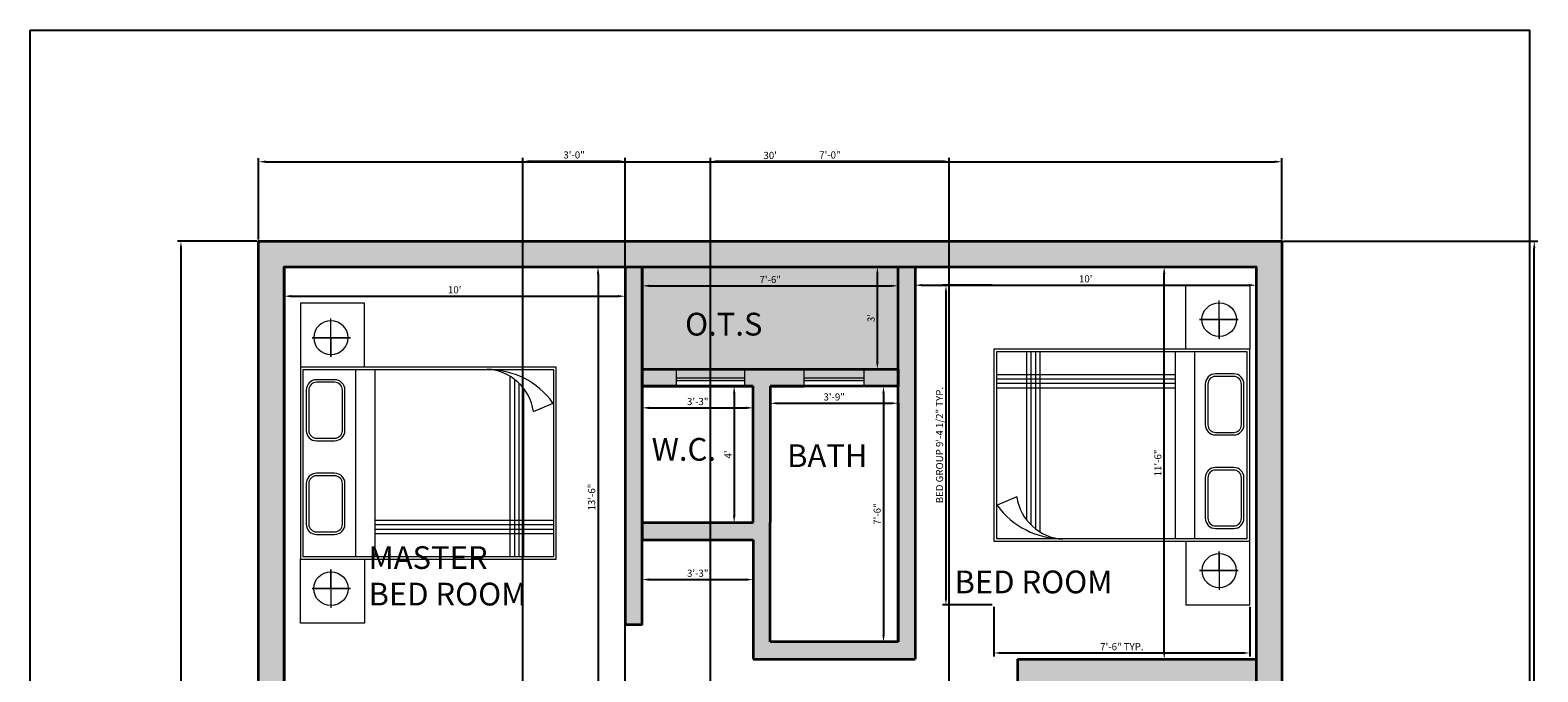
# Model space of a CAD drawing. Units: inches. Extents: x 2341 to 2872, y 1788 to 2419.
# Tile 3 of 3: x 2341 to 2872, y 2194 to 2419. Entities that reach past the tile are written whole.
import ezdxf

# ---------------------------------------------------------------- set-up
doc = ezdxf.new("R2010")
doc.units = ezdxf.units.IN
for name, color, linetype, lineweight in [('A-ANNO-DIMS', 2, 'Continuous', 18), ('A-ANNO-TTLB', 7, 'Continuous', 25), ('A-AREA-IDEN', 7, 'Continuous', 25), ('A-FURN', 8, 'Continuous', 18), ('A-GLAZ', 4, 'Continuous', 18), ('A-WALL', 7, 'Continuous', 35)]:
    doc.layers.add(name, color=color, linetype=linetype, lineweight=lineweight)
doc.layers.add('A-WALL-PATT', color=18, linetype='Continuous', lineweight=13, true_color=0x000000)
doc.styles.get("Standard").update_dxf_attribs({"font": 'arial.ttf'})
doc.dimstyles.new('Copy of ISO-25', dxfattribs={"dimtxt": 2.5, "dimasz": 2.5, "dimexe": 1.25, "dimexo": 0.625, "dimtad": 1, "dimdec": 1, "dimlunit": 4, "dimtxsty": 'Standard', "dimcen": 2.5, "dimadec": 0, "dimazin": 0, "dimtfac": 1, "dimtdec": 1, "dimtmove": 0, "dimatfit": 3, "dimfxl": 1, "dimarcsym": 0})

# ---------------------------------------------------------------- blocks, each defined once
blk = doc.blocks.new('*D1')
at = {"layer": 'A-ANNO-DIMS', "color": 0, "lineweight": -2, "transparency": 16777216}
for p, q in [((2421.55, 2345.64), (2421.55, 2374.26)), ((2424.05, 2373.01), (2779.05, 2373.01)), ((2781.55, 2345.64), (2781.55, 2374.26))]:
    blk.add_line(p, q, dxfattribs=at)
at = {"layer": 'A-ANNO-DIMS', "color": 0, "transparency": 16777216}
for points in [[(2424.05, 2373.43), (2424.05, 2372.6), (2421.55, 2373.01)], [(2779.05, 2373.43), (2779.05, 2372.6), (2781.55, 2373.01)]]:
    blk.add_solid(points, dxfattribs=at)
at = {"layer": 'Defpoints', "color": 0, "transparency": 16777216}
for p in [(2781.55, 2373.01), (2421.55, 2345.02), (2781.55, 2345.02)]:
    blk.add_point(p, dxfattribs=at)
at = {"layer": 'A-ANNO-DIMS', "color": 0, "transparency": 16777216, "insert": (2601.55, 2374.91), "char_height": 2.5, "attachment_point": 5}
blk.add_mtext("30'", dxfattribs=at)
blk = doc.blocks.new('A$C057D194F')
for p, q in [((0, 1.5, -0.169), (0, 2, -0.169)), ((0, 2, -0.169), (0.5, 2, -0.169)), ((0.269, 1.908, -0.169), (0.269, 1.761, -0.169)), ((0.269, 1.608, -0.169), (0.269, 1.908, -0.169)), ((0.5, 2, -0.169), (0.5, 0, -0.169)), ((2, 2, -0.169), (0.5, 2, -0.169)), ((1.98, 1.98, -0.169), (0.52, 1.98, -0.169)), ((0.52, 1.98, -0.169), (0.52, 0.02, -0.169)), ((1.091, 1.954, -0.169), (0.773, 1.954, -0.169)), ((1.091, 1.934, -0.169), (0.773, 1.934, -0.169)), ((1.822, 1.954, -0.169), (1.505, 1.954, -0.169)), ((1.822, 1.934, -0.169), (1.505, 1.934, -0.169)), ((1.98, 0.02, -0.169), (1.98, 1.98, -0.169)), ((2, 0, -0.169), (2, 2, -0.169)), ((2.5, 2, -0.169), (2, 2, -0.169)), ((2.231, 1.908, -0.169), (2.231, 1.761, -0.169)), ((2.231, 1.608, -0.169), (2.231, 1.908, -0.169)), ((2.5, 1.5, -0.169), (2.5, 2, -0.169)), ((0.693, 1.874, -0.169), (0.693, 1.732, -0.169)), ((0.713, 1.874, -0.169), (0.713, 1.732, -0.169)), ((1.151, 1.732, -0.169), (1.151, 1.874, -0.169)), ((1.171, 1.732, -0.169), (1.171, 1.874, -0.169)), ((1.425, 1.874, -0.169), (1.425, 1.732, -0.169)), ((1.445, 1.874, -0.169), (1.445, 1.732, -0.169)), ((1.882, 1.732, -0.169), (1.882, 1.874, -0.169)), ((1.902, 1.732, -0.169), (1.902, 1.874, -0.169)), ((0.419, 1.761, -0.169), (0.119, 1.761, -0.169)), ((0.269, 1.761, -0.169), (0.419, 1.761, -0.169)), ((0.269, 1.761, -0.169), (0.269, 1.608, -0.169)), ((0.773, 1.672, -0.169), (1.091, 1.672, -0.169)), ((0.773, 1.652, -0.169), (1.091, 1.652, -0.169)), ((1.505, 1.672, -0.169), (1.822, 1.672, -0.169)), ((1.505, 1.652, -0.169), (1.822, 1.652, -0.169)), ((2.081, 1.761, -0.169), (2.381, 1.761, -0.169)), ((2.231, 1.761, -0.169), (2.081, 1.761, -0.169)), ((2.231, 1.761, -0.169), (2.231, 1.608, -0.169)), ((1.98, 1.569, -0.169), (0.52, 1.569, -0.169)), ((0.5, 1.5, -0.169), (0, 1.5, -0.169)), ((1.98, 1.419, -0.169), (0.52, 1.419, -0.169)), ((0.697, 0.02, -0.169), (0.697, 1.419, -0.169)), ((0.732, 0.02, -0.169), (0.732, 1.419, -0.169)), ((0.767, 0.02, -0.169), (0.767, 1.419, -0.169)), ((0.802, 0.02, -0.169), (0.802, 1.419, -0.169)), ((2, 1.5, -0.169), (2.5, 1.5, -0.169)), ((0.52, 0.359, -0.169), (1.929, 0.359, -0.169)), ((0.52, 0.324, -0.169), (1.905, 0.324, -0.169)), ((0.52, 0.289, -0.169), (1.874, 0.289, -0.169)), ((0.52, 0.254, -0.169), (1.834, 0.254, -0.169)), ((1.655, 0.179, -0.169), (1.72, 0.025, -0.169)), ((0.52, 0.02, -0.169), (1.98, 0.02, -0.169)), ((0.5, 0, -0.169), (2, 0, -0.169))]:
    blk.add_line(p, q)
for centre, radius, start, end in [((0.773, 1.874, -0.169), 0.08, 90, 180), ((0.773, 1.874, -0.169), 0.06, 90, 180), ((1.091, 1.874, -0.169), 0.08, 0, 90), ((1.091, 1.874, -0.169), 0.06, 0, 90), ((1.505, 1.874, -0.169), 0.08, 90, 180), ((1.505, 1.874, -0.169), 0.06, 90, 180), ((1.822, 1.874, -0.169), 0.08, 0, 90), ((1.822, 1.874, -0.169), 0.06, 0, 90), ((0.773, 1.732, -0.169), 0.08, 180, 270), ((0.773, 1.732, -0.169), 0.06, 180, 270), ((1.091, 1.732, -0.169), 0.08, 270, 0), ((1.091, 1.732, -0.169), 0.06, 270, 0), ((1.505, 1.732, -0.169), 0.08, 180, 270), ((1.505, 1.732, -0.169), 0.06, 180, 270), ((1.822, 1.732, -0.169), 0.08, 270, 0), ((1.822, 1.732, -0.169), 0.06, 270, 0), ((1.599, 0.562, -0.169), 0.387, 278.2518, 356.6808), ((1.363, 0.529, -0.169), 0.617, 305.3295, 1.0459)]:
    blk.add_arc(centre, radius, start, end)
blk.add_ellipse((0.269, 1.761, -0.169), major_axis=(0, -0.135), ratio=0.975448)
at = {"extrusion": (0, 0, -1)}
blk.add_ellipse((2.231, 1.761, -0.169), major_axis=(0, 0.135), ratio=0.975448, dxfattribs=at)
for p in [(0.269, 1.761, -0.169), (2.231, 1.761, -0.169)]:
    blk.add_point(p)
blk = doc.blocks.new('*D4')
at = {"layer": 'A-ANNO-DIMS', "color": 0, "lineweight": -2, "transparency": 16777216}
for p, q in [((2420.93, 2345.02), (2392.99, 2345.02)), ((2394.24, 2342.52), (2394.24, 1987.52)), ((2420.93, 1985.02), (2392.99, 1985.02))]:
    blk.add_line(p, q, dxfattribs=at)
at = {"layer": 'A-ANNO-DIMS', "color": 0, "transparency": 16777216}
for points in [[(2393.82, 2342.52), (2394.66, 2342.52), (2394.24, 2345.02)], [(2393.82, 1987.52), (2394.66, 1987.52), (2394.24, 1985.02)]]:
    blk.add_solid(points, dxfattribs=at)
at = {"layer": 'Defpoints', "color": 0, "transparency": 16777216}
for p in [(2421.55, 2345.02), (2394.24, 1985.02), (2421.55, 1985.02)]:
    blk.add_point(p, dxfattribs=at)
at = {"layer": 'A-ANNO-DIMS', "color": 0, "transparency": 16777216, "insert": (2392.34, 2165.02), "char_height": 2.5, "attachment_point": 5, "rotation": 90}
blk.add_mtext("30'", dxfattribs=at)
blk = doc.blocks.new('*D7')
at = {"layer": 'A-ANNO-DIMS', "color": 0, "lineweight": -2, "transparency": 16777216}
for p, q in [((2430.55, 2335.39), (2430.55, 2324.45)), ((2550.55, 2335.39), (2550.55, 2324.45)), ((2433.05, 2325.7), (2548.05, 2325.7))]:
    blk.add_line(p, q, dxfattribs=at)
at = {"layer": 'A-ANNO-DIMS', "color": 0, "transparency": 16777216}
for points in [[(2433.05, 2326.12), (2433.05, 2325.29), (2430.55, 2325.7)], [(2548.05, 2326.12), (2548.05, 2325.29), (2550.55, 2325.7)]]:
    blk.add_solid(points, dxfattribs=at)
at = {"layer": 'Defpoints', "color": 0, "transparency": 16777216}
for p in [(2430.55, 2336.02), (2550.55, 2336.02), (2550.55, 2325.7)]:
    blk.add_point(p, dxfattribs=at)
at = {"layer": 'A-ANNO-DIMS', "color": 0, "transparency": 16777216, "insert": (2490.55, 2327.61), "char_height": 2.5, "attachment_point": 5}
blk.add_mtext("10'", dxfattribs=at)
blk = doc.blocks.new('*D8')
at = {"layer": 'A-ANNO-DIMS', "color": 0, "lineweight": -2, "transparency": 16777216}
for p, q in [((2549.93, 2336.02), (2539.72, 2336.02)), ((2540.97, 2333.52), (2540.97, 2176.52)), ((2549.93, 2174.02), (2539.72, 2174.02))]:
    blk.add_line(p, q, dxfattribs=at)
at = {"layer": 'A-ANNO-DIMS', "color": 0, "transparency": 16777216}
for points in [[(2540.56, 2333.52), (2541.39, 2333.52), (2540.97, 2336.02)], [(2540.56, 2176.52), (2541.39, 2176.52), (2540.97, 2174.02)]]:
    blk.add_solid(points, dxfattribs=at)
at = {"layer": 'Defpoints', "color": 0, "transparency": 16777216}
for p in [(2550.55, 2336.02), (2540.97, 2174.02), (2550.55, 2174.02)]:
    blk.add_point(p, dxfattribs=at)
at = {"layer": 'A-ANNO-DIMS', "color": 0, "transparency": 16777216, "insert": (2539.07, 2255.02), "char_height": 2.5, "attachment_point": 5, "rotation": 90}
blk.add_mtext('13\'-6"', dxfattribs=at)
blk = doc.blocks.new('*D9')
at = {"layer": 'A-ANNO-DIMS', "color": 0, "lineweight": -2, "transparency": 16777216}
for p, q in [((2556.55, 2335.39), (2556.55, 2328.09)), ((2646.55, 2335.39), (2646.55, 2328.09)), ((2559.05, 2329.34), (2644.05, 2329.34))]:
    blk.add_line(p, q, dxfattribs=at)
at = {"layer": 'A-ANNO-DIMS', "color": 0, "transparency": 16777216}
for points in [[(2559.05, 2329.76), (2559.05, 2328.93), (2556.55, 2329.34)], [(2644.05, 2329.76), (2644.05, 2328.93), (2646.55, 2329.34)]]:
    blk.add_solid(points, dxfattribs=at)
at = {"layer": 'Defpoints', "color": 0, "transparency": 16777216}
for p in [(2556.55, 2336.02), (2646.55, 2336.02), (2646.55, 2329.34)]:
    blk.add_point(p, dxfattribs=at)
at = {"layer": 'A-ANNO-DIMS', "color": 0, "transparency": 16777216, "insert": (2601.55, 2331.24), "char_height": 2.5, "attachment_point": 5}
blk.add_mtext('7\'-6"', dxfattribs=at)
blk = doc.blocks.new('*D10')
at = {"layer": 'A-ANNO-DIMS', "color": 0, "lineweight": -2, "transparency": 16777216}
for p, q in [((2645.93, 2336.02), (2638.01, 2336.02)), ((2639.26, 2302.52), (2639.26, 2333.52)), ((2645.93, 2300.02), (2638.01, 2300.02))]:
    blk.add_line(p, q, dxfattribs=at)
at = {"layer": 'A-ANNO-DIMS', "color": 0, "transparency": 16777216}
for points in [[(2638.84, 2333.52), (2639.67, 2333.52), (2639.26, 2336.02)], [(2638.84, 2302.52), (2639.67, 2302.52), (2639.26, 2300.02)]]:
    blk.add_solid(points, dxfattribs=at)
at = {"layer": 'Defpoints', "color": 0, "transparency": 16777216}
for p in [(2639.26, 2336.02), (2646.55, 2336.02), (2646.55, 2300.02)]:
    blk.add_point(p, dxfattribs=at)
at = {"layer": 'A-ANNO-DIMS', "color": 0, "transparency": 16777216, "insert": (2637.36, 2318.02), "char_height": 2.5, "attachment_point": 5, "rotation": 90}
blk.add_mtext("3'", dxfattribs=at)
blk = doc.blocks.new('*D11')
at = {"layer": 'A-ANNO-DIMS', "color": 0, "lineweight": -2, "transparency": 16777216}
for p, q in [((2601.55, 2293.39), (2601.55, 2286.77)), ((2646.55, 2293.39), (2646.55, 2286.77)), ((2604.05, 2288.02), (2644.05, 2288.02))]:
    blk.add_line(p, q, dxfattribs=at)
at = {"layer": 'A-ANNO-DIMS', "color": 0, "transparency": 16777216}
for points in [[(2604.05, 2288.43), (2604.05, 2287.6), (2601.55, 2288.02)], [(2644.05, 2288.43), (2644.05, 2287.6), (2646.55, 2288.02)]]:
    blk.add_solid(points, dxfattribs=at)
at = {"layer": 'Defpoints', "color": 0, "transparency": 16777216}
for p in [(2601.55, 2294.02), (2646.55, 2294.02), (2646.55, 2288.02)]:
    blk.add_point(p, dxfattribs=at)
at = {"layer": 'A-ANNO-DIMS', "color": 0, "transparency": 16777216, "insert": (2624.05, 2289.92), "char_height": 2.5, "attachment_point": 5}
blk.add_mtext('3\'-9"', dxfattribs=at)
blk = doc.blocks.new('*D12')
at = {"layer": 'A-ANNO-DIMS', "color": 0, "lineweight": -2, "transparency": 16777216}
for p, q in [((2645.93, 2294.02), (2640.16, 2294.02)), ((2641.41, 2291.52), (2641.41, 2206.52)), ((2645.93, 2204.02), (2640.16, 2204.02))]:
    blk.add_line(p, q, dxfattribs=at)
at = {"layer": 'A-ANNO-DIMS', "color": 0, "transparency": 16777216}
for points in [[(2640.99, 2291.52), (2641.82, 2291.52), (2641.41, 2294.02)], [(2640.99, 2206.52), (2641.82, 2206.52), (2641.41, 2204.02)]]:
    blk.add_solid(points, dxfattribs=at)
at = {"layer": 'Defpoints', "color": 0, "transparency": 16777216}
for p in [(2646.55, 2294.02), (2641.41, 2204.02), (2646.55, 2204.02)]:
    blk.add_point(p, dxfattribs=at)
at = {"layer": 'A-ANNO-DIMS', "color": 0, "transparency": 16777216, "insert": (2639.5, 2249.02), "char_height": 2.5, "attachment_point": 5, "rotation": 90}
blk.add_mtext('7\'-6"', dxfattribs=at)
blk = doc.blocks.new('*D13')
at = {"layer": 'A-ANNO-DIMS', "color": 0, "lineweight": -2, "transparency": 16777216}
for p, q in [((2556.55, 2293.39), (2556.55, 2285.16)), ((2595.55, 2293.39), (2595.55, 2285.16)), ((2559.05, 2286.41), (2593.05, 2286.41))]:
    blk.add_line(p, q, dxfattribs=at)
at = {"layer": 'A-ANNO-DIMS', "color": 0, "transparency": 16777216}
for points in [[(2559.05, 2286.83), (2559.05, 2285.99), (2556.55, 2286.41)], [(2593.05, 2286.83), (2593.05, 2285.99), (2595.55, 2286.41)]]:
    blk.add_solid(points, dxfattribs=at)
at = {"layer": 'Defpoints', "color": 0, "transparency": 16777216}
for p in [(2556.55, 2294.02), (2595.55, 2294.02), (2595.55, 2286.41)]:
    blk.add_point(p, dxfattribs=at)
at = {"layer": 'A-ANNO-DIMS', "color": 0, "transparency": 16777216, "insert": (2576.05, 2288.31), "char_height": 2.5, "attachment_point": 5}
blk.add_mtext('3\'-3"', dxfattribs=at)
blk = doc.blocks.new('*D14')
at = {"layer": 'A-ANNO-DIMS', "color": 0, "lineweight": -2, "transparency": 16777216}
for p, q in [((2594.93, 2294.02), (2587.63, 2294.02)), ((2588.88, 2291.52), (2588.88, 2248.52)), ((2594.93, 2246.02), (2587.63, 2246.02))]:
    blk.add_line(p, q, dxfattribs=at)
at = {"layer": 'A-ANNO-DIMS', "color": 0, "transparency": 16777216}
for points in [[(2588.46, 2291.52), (2589.3, 2291.52), (2588.88, 2294.02)], [(2588.46, 2248.52), (2589.3, 2248.52), (2588.88, 2246.02)]]:
    blk.add_solid(points, dxfattribs=at)
at = {"layer": 'Defpoints', "color": 0, "transparency": 16777216}
for p in [(2595.55, 2294.02), (2588.88, 2246.02), (2595.55, 2246.02)]:
    blk.add_point(p, dxfattribs=at)
at = {"layer": 'A-ANNO-DIMS', "color": 0, "transparency": 16777216, "insert": (2587.01, 2270.02), "char_height": 2.5, "attachment_point": 5, "rotation": 90}
blk.add_mtext("4'", dxfattribs=at)
blk = doc.blocks.new('*D15')
at = {"layer": 'A-ANNO-DIMS', "color": 0, "lineweight": -2, "transparency": 16777216}
for p, q in [((2652.55, 2335.39), (2652.55, 2328.32)), ((2772.55, 2335.39), (2772.55, 2328.32)), ((2655.05, 2329.57), (2770.05, 2329.57))]:
    blk.add_line(p, q, dxfattribs=at)
at = {"layer": 'A-ANNO-DIMS', "color": 0, "transparency": 16777216}
for points in [[(2655.05, 2329.98), (2655.05, 2329.15), (2652.55, 2329.57)], [(2770.05, 2329.98), (2770.05, 2329.15), (2772.55, 2329.57)]]:
    blk.add_solid(points, dxfattribs=at)
at = {"layer": 'Defpoints', "color": 0, "transparency": 16777216}
for p in [(2652.55, 2336.02), (2772.55, 2336.02), (2772.55, 2329.57)]:
    blk.add_point(p, dxfattribs=at)
at = {"layer": 'A-ANNO-DIMS', "color": 0, "transparency": 16777216, "insert": (2712.55, 2331.47), "char_height": 2.5, "attachment_point": 5}
blk.add_mtext("10'", dxfattribs=at)
blk = doc.blocks.new('*D16')
at = {"layer": 'A-ANNO-DIMS', "color": 0, "lineweight": -2, "transparency": 16777216}
for p, q in [((2771.93, 2336.02), (2738.91, 2336.02)), ((2740.16, 2200.52), (2740.16, 2333.52)), ((2771.93, 2198.02), (2738.91, 2198.02))]:
    blk.add_line(p, q, dxfattribs=at)
at = {"layer": 'A-ANNO-DIMS', "color": 0, "transparency": 16777216}
for points in [[(2739.74, 2333.52), (2740.58, 2333.52), (2740.16, 2336.02)], [(2739.74, 2200.52), (2740.58, 2200.52), (2740.16, 2198.02)]]:
    blk.add_solid(points, dxfattribs=at)
at = {"layer": 'Defpoints', "color": 0, "transparency": 16777216}
for p in [(2740.16, 2336.02), (2772.55, 2336.02), (2772.55, 2198.02)]:
    blk.add_point(p, dxfattribs=at)
at = {"layer": 'A-ANNO-DIMS', "color": 0, "transparency": 16777216, "insert": (2738.26, 2267.02), "char_height": 2.5, "attachment_point": 5, "rotation": 90}
blk.add_mtext('11\'-6"', dxfattribs=at)
blk = doc.blocks.new('*D29')
at = {"layer": 'A-ANNO-DIMS', "color": 0, "lineweight": -2, "transparency": 16777216}
for p, q in [((2556.55, 2239.39), (2556.55, 2224.73)), ((2595.55, 2239.39), (2595.55, 2224.73)), ((2559.05, 2225.98), (2593.05, 2225.98))]:
    blk.add_line(p, q, dxfattribs=at)
at = {"layer": 'A-ANNO-DIMS', "color": 0, "transparency": 16777216}
for points in [[(2559.05, 2226.4), (2559.05, 2225.56), (2556.55, 2225.98)], [(2593.05, 2226.4), (2593.05, 2225.56), (2595.55, 2225.98)]]:
    blk.add_solid(points, dxfattribs=at)
at = {"layer": 'Defpoints', "color": 0, "transparency": 16777216}
for p in [(2556.55, 2240.02), (2595.55, 2240.02), (2595.55, 2225.98)]:
    blk.add_point(p, dxfattribs=at)
at = {"layer": 'A-ANNO-DIMS', "color": 0, "transparency": 16777216, "insert": (2576.05, 2227.88), "char_height": 2.5, "attachment_point": 5}
blk.add_mtext('3\'-3"', dxfattribs=at)
blk = doc.blocks.new('*D31')
at = {"layer": 'A-ANNO-DIMS', "color": 0, "lineweight": -2, "transparency": 16777216}
for p, q in [((2679.63, 2329.57), (2662.13, 2329.57)), ((2663.38, 2327.07), (2663.38, 2219.54)), ((2679.63, 2217.04), (2662.13, 2217.04))]:
    blk.add_line(p, q, dxfattribs=at)
at = {"layer": 'A-ANNO-DIMS', "color": 0, "transparency": 16777216}
for points in [[(2662.96, 2327.07), (2663.79, 2327.07), (2663.38, 2329.57)], [(2662.96, 2219.54), (2663.79, 2219.54), (2663.38, 2217.04)]]:
    blk.add_solid(points, dxfattribs=at)
at = {"layer": 'Defpoints', "color": 0, "transparency": 16777216}
for p in [(2680.26, 2329.57), (2663.38, 2217.04), (2680.26, 2217.04)]:
    blk.add_point(p, dxfattribs=at)
at = {"layer": 'A-ANNO-DIMS', "color": 0, "transparency": 16777216, "insert": (2661.46, 2273.3), "char_height": 2.5, "attachment_point": 5, "rotation": 90}
blk.add_mtext('BED GROUP 9\'-4 1/2" TYP.', dxfattribs=at)
blk = doc.blocks.new('*D32')
at = {"layer": 'A-ANNO-DIMS', "color": 0, "lineweight": -2, "transparency": 16777216}
for p, q in [((2680.26, 2216.41), (2680.26, 2198.91)), ((2770.28, 2216.41), (2770.28, 2198.91)), ((2682.76, 2200.16), (2767.78, 2200.16))]:
    blk.add_line(p, q, dxfattribs=at)
at = {"layer": 'A-ANNO-DIMS', "color": 0, "transparency": 16777216}
for points in [[(2682.76, 2200.57), (2682.76, 2199.74), (2680.26, 2200.16)], [(2767.78, 2200.57), (2767.78, 2199.74), (2770.28, 2200.16)]]:
    blk.add_solid(points, dxfattribs=at)
at = {"layer": 'Defpoints', "color": 0, "transparency": 16777216}
for p in [(2680.26, 2217.04), (2770.28, 2217.04), (2770.28, 2200.16)]:
    blk.add_point(p, dxfattribs=at)
at = {"layer": 'A-ANNO-DIMS', "color": 0, "transparency": 16777216, "insert": (2725.27, 2202.06), "char_height": 2.5, "attachment_point": 5}
blk.add_mtext('7\'-6" TYP.', dxfattribs=at)
blk = doc.blocks.new('*D35')
at = {"layer": 'A-ANNO-DIMS', "color": 0, "lineweight": -2, "transparency": 16777216}
for p, q in [((2782.18, 2345.02), (2871.62, 2345.02)), ((2870.37, 1945.52), (2870.37, 2342.52)), ((2782.18, 1943.02), (2871.62, 1943.02))]:
    blk.add_line(p, q, dxfattribs=at)
at = {"layer": 'A-ANNO-DIMS', "color": 0, "transparency": 16777216}
for points in [[(2869.95, 2342.52), (2870.78, 2342.52), (2870.37, 2345.02)], [(2869.95, 1945.52), (2870.78, 1945.52), (2870.37, 1943.02)]]:
    blk.add_solid(points, dxfattribs=at)
at = {"layer": 'Defpoints', "color": 0, "transparency": 16777216}
for p in [(2781.55, 2345.02), (2870.37, 2345.02), (2781.55, 1943.02)]:
    blk.add_point(p, dxfattribs=at)
at = {"layer": 'A-ANNO-DIMS', "color": 0, "transparency": 16777216, "insert": (2868.46, 2144.02), "char_height": 2.5, "attachment_point": 5, "rotation": 90}
blk.add_mtext('33\'-6"', dxfattribs=at)
blk = doc.blocks.new('*D37')
at = {"layer": 'A-ANNO-DIMS', "color": 0, "lineweight": -2, "transparency": 16777216}
for p, q in [((2580.55, 2120.64), (2580.55, 2374.42)), ((2583.05, 2373.17), (2662.05, 2373.17)), ((2664.55, 2120.64), (2664.55, 2374.42))]:
    blk.add_line(p, q, dxfattribs=at)
at = {"layer": 'A-ANNO-DIMS', "color": 0, "transparency": 16777216}
for points in [[(2583.05, 2373.58), (2583.05, 2372.75), (2580.55, 2373.17)], [(2662.05, 2373.58), (2662.05, 2372.75), (2664.55, 2373.17)]]:
    blk.add_solid(points, dxfattribs=at)
at = {"layer": 'Defpoints', "color": 0, "transparency": 16777216}
for p in [(2664.55, 2373.17), (2580.55, 2120.02), (2664.55, 2120.02)]:
    blk.add_point(p, dxfattribs=at)
at = {"layer": 'A-ANNO-DIMS', "color": 0, "transparency": 16777216, "insert": (2622.55, 2375.07), "char_height": 2.5, "attachment_point": 5}
blk.add_mtext('7\'-0"', dxfattribs=at)
blk = doc.blocks.new('*D38')
at = {"layer": 'A-ANNO-DIMS', "color": 0, "lineweight": -2, "transparency": 16777216}
for p, q in [((2514.55, 2120.64), (2514.55, 2374.42)), ((2517.05, 2373.17), (2548.05, 2373.17)), ((2550.55, 2120.64), (2550.55, 2374.42))]:
    blk.add_line(p, q, dxfattribs=at)
at = {"layer": 'A-ANNO-DIMS', "color": 0, "transparency": 16777216}
for points in [[(2517.05, 2373.58), (2517.05, 2372.75), (2514.55, 2373.17)], [(2548.05, 2373.58), (2548.05, 2372.75), (2550.55, 2373.17)]]:
    blk.add_solid(points, dxfattribs=at)
at = {"layer": 'Defpoints', "color": 0, "transparency": 16777216}
for p in [(2550.55, 2373.17), (2514.55, 2120.02), (2550.55, 2120.02)]:
    blk.add_point(p, dxfattribs=at)
at = {"layer": 'A-ANNO-DIMS', "color": 0, "transparency": 16777216, "insert": (2532.55, 2375.07), "char_height": 2.5, "attachment_point": 5}
blk.add_mtext('3\'-0"', dxfattribs=at)

msp = doc.modelspace()

# ---------------------------------------------------------------- hatches: boundary and pattern name
at = {"layer": 'A-WALL-PATT'}
h = msp.add_hatch(color=256, dxfattribs=at)
h.dxf.hatch_style = 1
h.paths.add_polyline_path([(2781.55, 2345.02), (2421.55, 2345.02), (2421.55, 1985.02), (2421.55, 1949.02), (2421.55, 1943.02), (2781.55, 1943.02), (2781.55, 1985.02)])
h.paths.add_polyline_path([(2550.55, 2336.02), (2772.55, 2336.02), (2772.55, 1994.02), (2772.55, 1985.02), (2772.55, 1947.02), (2430.55, 1947.02), (2430.55, 1985.02), (2454.55, 1985.02), (2454.55, 1994.02), (2430.55, 1994.02), (2430.55, 2114.02), (2496.55, 2114.02), (2514.55, 2114.02), (2514.55, 2120.02), (2496.55, 2120.02), (2496.55, 2168.02), (2556.55, 2168.02), (2556.55, 2174.02), (2550.55, 2174.02), (2478.55, 2174.02), (2478.55, 2170.02), (2490.55, 2170.02), (2490.55, 2168.02), (2490.55, 2120.02), (2430.55, 2120.02), (2430.55, 2168.02), (2430.55, 2174.02), (2430.55, 2204.02), (2430.55, 2336.02)], flags=16)
h.paths.add_polyline_path([(2556.55, 2336.02), (2652.55, 2336.02), (2652.55, 2198.02), (2646.55, 2198.02), (2601.55, 2198.02), (2595.55, 2198.02), (2595.55, 2240.02), (2556.55, 2240.02), (2556.55, 2246.02), (2556.55, 2294.02)], flags=0)
h.paths.add_polyline_path([(2556.55, 2300.02), (2646.55, 2300.02), (2646.55, 2294.02), (2646.55, 2204.02), (2601.55, 2204.02), (2601.55, 2246.02), (2601.55, 2294.02), (2613.55, 2294.02), (2613.55, 2300.02), (2592.55, 2300.02), (2592.55, 2294.02), (2595.55, 2294.02), (2595.55, 2246.02), (2556.55, 2246.02), (2556.55, 2282.02)], flags=0)
h.paths.add_polyline_path([(2680.26, 2307.06), (2747.77, 2307.06), (2747.77, 2329.57), (2770.28, 2329.57), (2770.28, 2307.06), (2770.28, 2239.54), (2770.28, 2217.04), (2747.77, 2217.04), (2747.77, 2239.54), (2680.26, 2239.54)], flags=0)
h.paths.add_polyline_path([(2681.16, 2306.16), (2769.38, 2306.16), (2769.38, 2240.44), (2704.56, 2240.44, -0.009128), (2703.54, 2240.44), (2681.16, 2240.44)], flags=0)
h.paths.add_polyline_path([(2744.14, 2298.19), (2744.14, 2293.47), (2696.44, 2293.47), (2696.44, 2242.73, -0.092104), (2691.71, 2247), (2691.71, 2298.19)], flags=0)
h.paths.add_polyline_path([(2694.86, 2296.62), (2694.86, 2295.04), (2693.29, 2295.04), (2693.29, 2296.62)], flags=0)
h.paths.add_polyline_path([(2478.55, 2173.02), (2478.55, 2172.02), (2478.55, 2171.02), (2442.55, 2171.02), (2442.55, 2170.02), (2438.98, 2170.02), (2430.55, 2170.02), (2430.55, 2174.02), (2442.55, 2174.02), (2442.55, 2173.02)], flags=0)
h.paths.add_polyline_path([(2688.55, 2198.02), (2697.55, 2198.02), (2772.55, 2198.02), (2772.55, 2189.02), (2772.55, 2153.02), (2755.26, 2153.02), (2755.26, 2145.02), (2772.55, 2145.02), (2772.55, 2137.02), (2755.26, 2137.02), (2755.26, 2129.02), (2772.55, 2129.02), (2772.55, 2121.02), (2755.26, 2121.02), (2755.26, 2119.07), (2757.66, 2119.07), (2755.26, 2113.02), (2772.55, 2113.02), (2772.55, 2105.02), (2736.55, 2105.02), (2736.55, 2153.02), (2697.55, 2153.02), (2697.55, 2021.02), (2697.55, 1952.02), (2688.89, 1952.02), (2688.89, 1947.02), (2688.59, 2021.02), (2688.55, 2021.02), (2580.55, 2021.02), (2580.55, 2030.02), (2556.55, 2030.02), (2556.55, 2114.02), (2580.55, 2114.02), (2580.55, 2120.02), (2664.55, 2120.02), (2688.55, 2120.02), (2688.55, 2189.02)], flags=0)
h.paths.add_polyline_path([(2510.86, 2109.17, -0.414214), (2512.75, 2107.25), (2512.59, 2085.13, -0.414214), (2511.43, 2083.99), (2508, 2084.02, -0.414214), (2506.86, 2085.17), (2487.78, 2085.31, -0.414214), (2485.88, 2087.24, -0.414214), (2483.96, 2085.34), (2464.87, 2085.49, -0.414214), (2462.98, 2087.41, -0.414214), (2461.06, 2085.52), (2441.97, 2085.66, -0.414214), (2440.82, 2084.52), (2437.38, 2084.55, -0.414214), (2436.25, 2085.7), (2436.41, 2107.83, -0.414214), (2438.34, 2109.72)], flags=0)
h.paths.add_polyline_path([(2736.55, 2189.02), (2736.55, 2170), (2728.55, 2170), (2728.55, 2153.02), (2720.55, 2153.02), (2720.55, 2189.02), (2712.55, 2189.02), (2712.55, 2153.02), (2704.55, 2153.02), (2704.55, 2189.02)], flags=0)
edge = h.paths.add_edge_path(flags=0)
edge.add_ellipse((2759.52, 2317.47), major_axis=(6.08, 0), ratio=0.975448, start_angle=450, end_angle=540, ccw=False)
edge.add_ellipse((2759.52, 2317.47), major_axis=(6.08, 0), ratio=0.975448, start_angle=360, end_angle=450, ccw=False)
edge.add_ellipse((2759.52, 2317.47), major_axis=(6.08, 0), ratio=0.975448, start_angle=270, end_angle=360, ccw=False)
edge.add_ellipse((2759.52, 2317.47), major_axis=(6.08, 0), ratio=0.975448, start_angle=180, end_angle=270, ccw=False)
h.paths.add_polyline_path([(2505.86, 2104.26, -0.414214), (2507, 2103.11), (2506.89, 2089.02), (2442, 2089.51), (2442.11, 2103.6, -0.414214), (2443.26, 2104.74)], flags=0)
h.paths.add_polyline_path([(2485.9, 2089.94), (2463, 2090.11), (2463.01, 2091.64), (2485.91, 2091.47)], flags=0)
h.paths.add_polyline_path([(2758.23, 2298.35), (2764.61, 2298.35, -0.414214), (2768.21, 2294.75), (2768.21, 2280.47, -0.414214), (2764.61, 2276.87), (2758.23, 2276.87, -0.414214), (2754.62, 2280.47), (2754.62, 2294.75, -0.414214)], flags=0)
h.paths.add_polyline_path([(2758.23, 2297.45), (2764.61, 2297.45, -0.414214), (2767.31, 2294.75), (2767.31, 2280.47, -0.414214), (2764.61, 2277.77), (2758.23, 2277.77, -0.414214), (2755.52, 2280.47), (2755.52, 2294.75, -0.414214)], flags=0)
h.paths.add_polyline_path([(2758.23, 2265.42), (2764.61, 2265.42, -0.414214), (2768.21, 2261.82), (2768.21, 2247.53, -0.414214), (2764.61, 2243.93), (2758.23, 2243.93, -0.414214), (2754.62, 2247.53), (2754.62, 2261.82, -0.414214)], flags=0)
h.paths.add_polyline_path([(2758.23, 2264.52), (2764.61, 2264.52, -0.414214), (2767.31, 2261.82), (2767.31, 2247.53, -0.414214), (2764.61, 2244.83), (2758.23, 2244.83, -0.414214), (2755.52, 2247.53), (2755.52, 2261.82, -0.414214)], flags=0)
edge = h.paths.add_edge_path(flags=0)
edge.add_ellipse((2759.52, 2229.13), major_axis=(6.08, 0), ratio=0.975448, start_angle=90, end_angle=180, ccw=False)
edge.add_ellipse((2759.52, 2229.13), major_axis=(6.08, 0), ratio=0.975448, start_angle=0, end_angle=90, ccw=False)
edge.add_ellipse((2759.52, 2229.13), major_axis=(6.08, 0), ratio=0.975448, start_angle=270, end_angle=360, ccw=False)
edge.add_ellipse((2759.52, 2229.13), major_axis=(6.08, 0), ratio=0.975448, start_angle=180, end_angle=270, ccw=False)
h.paths.add_polyline_path([(2457.94, 2073.59, -0.414214), (2459.08, 2072.44), (2459.05, 2069, -0.414214), (2457.9, 2067.87), (2457.75, 2048.78, -0.414214), (2455.83, 2046.89, -0.414214), (2457.72, 2044.96), (2457.58, 2025.88, -0.414214), (2455.66, 2023.98, -0.414214), (2457.55, 2022.06), (2457.41, 2002.98, -0.414214), (2458.54, 2001.82), (2458.52, 1998.39, -0.414214), (2457.36, 1997.25), (2435.24, 1997.42, -0.414214), (2433.35, 1999.34), (2433.89, 2071.86, -0.414214), (2435.82, 2073.76)], flags=0)
h.paths.add_polyline_path([(2454.05, 2067.89), (2453.56, 2003), (2439.47, 2003.11, -0.414214), (2438.33, 2004.26), (2438.8, 2066.86, -0.414214), (2439.96, 2068)], flags=0)
h.paths.add_polyline_path([(2452.95, 2024), (2451.43, 2024.02), (2451.6, 2046.92), (2453.13, 2046.91)], flags=0)
h.paths.add_polyline_path([(2830.4, 1819.46), (2838.99, 1819.46), (2838.99, 1828.46), (2830.4, 1828.46)], flags=9)
h.paths.add_polyline_path([(2814.93, 1841.19), (2823.62, 1841.19), (2823.62, 1850.5), (2814.93, 1850.5)], flags=9)
h.paths.add_polyline_path([(2843.19, 1840.36), (2852.25, 1840.36), (2852.25, 1849.36), (2843.19, 1849.36)], flags=9)
h.paths.add_polyline_path([(2828.19, 1854.15), (2839.1, 1854.15), (2839.1, 1863.15), (2828.19, 1863.15)], flags=9)
h.paths.add_polyline_path([(2760.12, 1830.89), (2792.1, 1830.89), (2792.1, 1840.21), (2760.12, 1840.21)], flags=9)
h.paths.add_polyline_path([(2760.12, 1840.53), (2800.48, 1840.53), (2800.48, 1849.85), (2760.12, 1849.85)], flags=9)
h.paths.add_polyline_path([(2758.73, 1854.24), (2815.82, 1854.24), (2815.82, 1863.56), (2758.73, 1863.56)], flags=9)
h.paths.add_polyline_path([(2482.08, 1917.73), (2536.72, 1917.73), (2536.72, 1936.36), (2482.08, 1936.36)], flags=9)
h.paths.add_polyline_path([(2707.72, 1951.32), (2770.13, 1951.32), (2770.13, 1963.73), (2707.72, 1963.73)], flags=8)
h.paths.add_polyline_path([(2706.05, 2121.97), (2725.65, 2121.97), (2725.65, 2134.17), (2706.05, 2134.17)], flags=8)
h.paths.add_polyline_path([(2705.12, 1972.11), (2749.62, 1972.11), (2749.62, 1984.52), (2705.12, 1984.52)], flags=8)
h.paths.add_polyline_path([(2468.66, 1961.36), (2524.36, 1961.36), (2524.36, 1973.77), (2468.66, 1973.77)], flags=8)
h.paths.add_polyline_path([(2572.95, 1988.2), (2639.05, 1988.2), (2639.05, 2000.2), (2572.95, 2000.2)], flags=8)
h.paths.add_polyline_path([(2460.85, 2050.66), (2556.87, 2050.66), (2556.87, 2063.08), (2460.85, 2063.08)], flags=8)
h.paths.add_polyline_path([(2575.44, 2073.64), (2628.63, 2073.64), (2628.63, 2086.04), (2575.44, 2086.04)], flags=8)
h.paths.add_polyline_path([(2575.12, 2153.95), (2616.53, 2153.95), (2616.53, 2166.37), (2575.12, 2166.37)], flags=8)
h.paths.add_polyline_path([(2664.33, 2218.95), (2729.32, 2218.95), (2729.32, 2231.37), (2664.33, 2231.37)], flags=8)
h.paths.add_polyline_path([(2557.77, 2265.61), (2586.74, 2265.61), (2586.74, 2278.02), (2557.77, 2278.02)], flags=8)
h.paths.add_polyline_path([(2605.48, 2263.57), (2639.29, 2263.57), (2639.29, 2275.57), (2605.48, 2275.57)], flags=8)
h.paths.add_polyline_path([(2569.54, 2309.66), (2602.87, 2309.66), (2602.87, 2322.07), (2569.54, 2322.07)], flags=8)
h.paths.add_polyline_path([(2458.16, 2214.67), (2523.15, 2214.67), (2523.15, 2227.09), (2458.16, 2227.09)], flags=8)
h.paths.add_polyline_path([(2458.16, 2227.52), (2511.98, 2227.52), (2511.98, 2239.93), (2458.16, 2239.93)], flags=8)
h.paths.add_polyline_path([(2449.57, 2140.97), (2449.57, 2149.18), (2444.42, 2149.18), (2444.42, 2140.97)], flags=8)
h.paths.add_polyline_path([(2458.63, 2128.07), (2462.49, 2128.07), (2462.49, 2133.23), (2458.63, 2133.23)], flags=8)
h.paths.add_polyline_path([(2506.29, 2142.15), (2506.29, 2146.01), (2501.14, 2146.01), (2501.14, 2142.15)], flags=8)
h.paths.add_polyline_path([(2487.54, 2002.8), (2493.34, 2002.8), (2493.34, 2007.95), (2487.54, 2007.95)], flags=8)
h.paths.add_polyline_path([(2479.27, 2051.01), (2479.27, 2056.81), (2474.12, 2056.81), (2474.12, 2051.01)], flags=8)
h.paths.add_polyline_path([(2441.47, 1961.92), (2441.47, 1970.13), (2436.31, 1970.13), (2436.31, 1961.92)], flags=8)
h.paths.add_polyline_path([(2682.8, 1979.93), (2682.8, 1988.13), (2677.65, 1988.13), (2677.65, 1979.93)], flags=8)
h.paths.add_polyline_path([(2752.63, 2088.44), (2756.49, 2088.44), (2756.49, 2093.6), (2752.63, 2093.6)], flags=8)
h.paths.add_polyline_path([(2752.63, 2180.4), (2756.49, 2180.4), (2756.49, 2185.55), (2752.63, 2185.55)], flags=8)
h.paths.add_polyline_path([(2740.86, 2261.83), (2740.86, 2271.98), (2735.71, 2271.98), (2735.71, 2261.83)], flags=8)
h.paths.add_polyline_path([(2709.54, 2328.87), (2715.34, 2328.87), (2715.34, 2334.02), (2709.54, 2334.02)], flags=8)
h.paths.add_polyline_path([(2639.95, 2316.1), (2639.95, 2319.95), (2634.8, 2319.95), (2634.8, 2316.1)], flags=8)
h.paths.add_polyline_path([(2597.45, 2328.64), (2605.65, 2328.64), (2605.65, 2333.8), (2597.45, 2333.8)], flags=8)
h.paths.add_polyline_path([(2487.54, 2325.01), (2493.34, 2325.01), (2493.34, 2330.16), (2487.54, 2330.16)], flags=8)
h.paths.add_polyline_path([(2541.67, 2249.83), (2541.67, 2259.98), (2536.52, 2259.98), (2536.52, 2249.83)], flags=8)
h = msp.add_hatch(color=256, dxfattribs=at)
h.dxf.hatch_style = 1
h.paths.add_polyline_path([(2556.55, 1994.02), (2556.55, 2021.02), (2580.55, 2021.02), (2580.55, 2030.02), (2556.55, 2030.02), (2556.55, 2114.02), (2580.55, 2114.02), (2580.55, 2120.02), (2556.55, 2120.02), (2550.55, 2120.02), (2550.55, 2114.02), (2550.55, 1994.02), (2526.55, 1994.02), (2526.55, 1985.02), (2556.55, 1985.02)])
h.paths.add_polyline_path([(2697.55, 2120.02), (2688.55, 2120.02), (2664.55, 2120.02), (2664.55, 2114.02), (2688.55, 2114.02), (2688.55, 2030.02), (2664.55, 2030.02), (2664.55, 2021.02), (2688.55, 2021.02), (2688.59, 2021.02), (2688.87, 1952.02), (2697.55, 1952.02), (2697.55, 2021.02)])
h.paths.add_polyline_path([(2772.55, 2198.02), (2688.55, 2198.02), (2688.55, 2189.02), (2688.55, 2153.02), (2697.55, 2153.02), (2697.55, 2189.02), (2772.55, 2189.02)])
h.paths.add_polyline_path([(2652.55, 2336.02), (2646.55, 2336.02), (2646.55, 2204.02), (2601.55, 2204.02), (2601.55, 2246.02), (2601.55, 2294.02), (2613.55, 2294.02), (2613.55, 2296.02), (2634.55, 2296.02), (2634.55, 2294.02), (2646.55, 2294.02), (2646.55, 2300.02), (2646.55, 2336.02), (2556.55, 2336.02), (2556.55, 2294.02), (2568.55, 2294.02), (2568.55, 2296.02), (2592.55, 2296.02), (2592.55, 2294.02), (2595.55, 2294.02), (2595.55, 2246.02), (2556.55, 2246.02), (2556.55, 2240.02), (2595.55, 2240.02), (2595.55, 2198.02), (2601.55, 2198.02), (2646.55, 2198.02), (2652.55, 2198.02)])
h.paths.add_polyline_path([(2442.55, 2174.02), (2430.55, 2174.02), (2430.55, 2170.02), (2442.55, 2170.02)])
h.paths.add_polyline_path([(2478.55, 2172.02), (2478.55, 2173.02), (2442.55, 2173.02), (2442.55, 2171.02), (2478.55, 2171.02)])
h.paths.add_polyline_path([(2556.55, 2336.02), (2550.55, 2336.02), (2550.55, 2210.02), (2556.55, 2210.02)])
h.paths.add_polyline_path([(2460.85, 2050.66), (2556.87, 2050.66), (2556.87, 2063.08), (2460.85, 2063.08)], flags=9)
h.paths.add_polyline_path([(2569.54, 2309.66), (2602.87, 2309.66), (2602.87, 2322.07), (2569.54, 2322.07)], flags=24)

# ---------------------------------------------------------------- linework, layer by layer
at = {"layer": 'A-ANNO-TTLB'}
msp.add_lwpolyline([(2341.19, 2419.31), (2868.69, 2419.31), (2868.69, 1813.17), (2341.19, 1813.17)], close=True, dxfattribs=at)
at = {"layer": 'A-GLAZ'}
for p, q in [((2568.55, 2294.02), (2568.55, 2300.02)), ((2568.55, 2300.02), (2580.55, 2300.02)), ((2568.55, 2300.02), (2592.55, 2300.02)), ((2568.55, 2297.02), (2592.55, 2297.02)), ((2580.55, 2300.02), (2592.55, 2300.02)), ((2592.55, 2300.02), (2592.55, 2294.02)), ((2613.55, 2294.02), (2613.55, 2300.02)), ((2613.55, 2297.02), (2634.55, 2297.02)), ((2634.55, 2294.02), (2634.55, 2300.02)), ((2568.55, 2296.02), (2592.55, 2296.02)), ((2613.55, 2296.02), (2634.55, 2296.02))]:
    msp.add_line(p, q, dxfattribs=at)
at = {"layer": 'A-WALL'}
for p, q in [((2781.55, 2345.02), (2781.55, 1985.02)), ((2430.55, 2336.02), (2550.55, 2336.02)), ((2430.55, 2336.02), (2430.55, 2204.02)), ((2550.55, 2336.02), (2550.55, 2210.02)), ((2556.55, 2336.02), (2652.55, 2336.02)), ((2556.55, 2336.02), (2556.55, 2288.02)), ((2556.55, 2336.02), (2556.55, 2300.02)), ((2556.55, 2210.02), (2556.55, 2336.02)), ((2646.55, 2204.02), (2646.55, 2336.02)), ((2652.55, 2336.02), (2652.55, 2198.02)), ((2556.55, 2300.02), (2646.55, 2300.02)), ((2646.55, 2300.02), (2646.55, 2294.02)), ((2556.55, 2294.02), (2556.55, 2246.02)), ((2556.55, 2294.02), (2556.55, 2294.02)), ((2556.55, 2294.02), (2595.55, 2294.02)), ((2595.55, 2294.02), (2556.55, 2294.02)), ((2556.55, 2294.02), (2568.55, 2294.02)), ((2595.55, 2246.02), (2595.55, 2294.02)), ((2646.55, 2294.02), (2601.55, 2294.02)), ((2601.55, 2294.02), (2601.55, 2246.02)), ((2601.55, 2294.02), (2613.55, 2294.02)), ((2646.55, 2294.02), (2634.55, 2294.02)), ((2646.55, 2288.02), (2646.55, 2282.02)), ((2556.55, 2282.02), (2556.55, 2275.04)), ((2556.55, 2282.02), (2556.55, 2246.02)), ((2646.55, 2282.02), (2646.55, 2204.02)), ((2556.55, 2246.02), (2556.55, 2240.02)), ((2556.55, 2246.02), (2595.55, 2246.02)), ((2556.55, 2246.02), (2556.55, 2240.02)), ((2601.55, 2204.02), (2601.55, 2246.02)), ((2556.55, 2240.02), (2595.55, 2240.02)), ((2595.55, 2240.02), (2595.55, 2198.02)), ((2556.55, 2210.02), (2550.55, 2210.02)), ((2430.55, 2204.02), (2430.55, 2174.02)), ((2646.55, 2204.02), (2601.55, 2204.02)), ((2595.55, 2198.02), (2601.55, 2198.02)), ((2601.55, 2198.02), (2646.55, 2198.02)), ((2646.55, 2198.02), (2652.55, 2198.02)), ((2688.55, 2198.02), (2772.55, 2198.02)), ((2688.55, 2198.02), (2688.55, 2189.02)), ((2688.55, 2198.02), (2697.55, 2198.02)), ((2772.55, 2198.02), (2772.55, 2189.02))]:
    msp.add_line(p, q, dxfattribs=at)
for points in [[(2421.55, 1985.02), (2421.55, 2345.02), (2781.55, 2345.02), (2781.55, 1985.02)], [(2430.55, 2174.02), (2430.55, 2336.02), (2772.55, 2336.02), (2772.55, 1994.02)]]:
    msp.add_lwpolyline(points, dxfattribs=at)

# ---------------------------------------------------------------- block references
at = {"layer": 'A-FURN', "xscale": 45.0119455694804, "yscale": 45.0119455694804, "zscale": 45.0119455694804}
for p, rotation in [((2680.26, 2329.57, 7.6), 270), ((2680.26, 2329.57, 7.6), 270), ((2526.28, 2210.68, 7.6), 89.99999999999999)]:
    msp.add_blockref('A$C057D194F', p, dxfattribs=dict(at, rotation=rotation))

# ---------------------------------------------------------------- texts
at = {"layer": 'A-AREA-IDEN'}
for s, p in [('O.T.S', (2571.61, 2311.86)), ('W.C.', (2559.84, 2267.81)), ('BATH', (2607.48, 2265.57)), ('MASTER ', (2460.23, 2229.73)), ('BED ROOM', (2666.4, 2221.16)), ('BED ROOM', (2460.23, 2216.88))]:
    msp.add_text(s, height=8, dxfattribs=at).set_placement(p)

# ---------------------------------------------------------------- dimensions: what is measured, and where the dimension line sits
at = {"layer": 'A-ANNO-DIMS'}
for base, p1, p2, override, picture, middle in [((2781.55, 2373.01), (2421.55, 2345.02), (2781.55, 2345.02), {"dimclrd": 0, "dimclre": 0, "dimclrt": 0}, '*D1', (2601.55, 2374.91)), ((2550.55, 2373.17), (2514.55, 2120.02), (2550.55, 2120.02), {"dimdec": 1, "dimlfac": 1, "dimrnd": 0, "dimzin": 1, "dimdsep": 46, "dimlunit": 4, "dimfrac": 2}, '*D38', (2532.55, 2375.07)), ((2664.55, 2373.17), (2580.55, 2120.02), (2664.55, 2120.02), {"dimdec": 1, "dimlfac": 1, "dimrnd": 0, "dimzin": 1, "dimdsep": 46, "dimlunit": 4, "dimfrac": 2}, '*D37', (2622.55, 2375.07)), ((2550.55, 2325.7), (2430.55, 2336.02), (2550.55, 2336.02), {"dimclrd": 0, "dimclre": 0, "dimclrt": 0}, '*D7', (2490.55, 2327.61)), ((2646.55, 2329.34), (2556.55, 2336.02), (2646.55, 2336.02), {"dimclrd": 0, "dimclre": 0, "dimclrt": 0}, '*D9', (2601.55, 2331.24)), ((2772.55, 2329.57), (2652.55, 2336.02), (2772.55, 2336.02), {"dimclrd": 0, "dimclre": 0, "dimclrt": 0}, '*D15', (2712.55, 2331.47)), ((2595.55, 2286.41), (2556.55, 2294.02), (2595.55, 2294.02), {"dimclrd": 0, "dimclre": 0, "dimclrt": 0}, '*D13', (2576.05, 2288.31)), ((2646.55, 2288.02), (2601.55, 2294.02), (2646.55, 2294.02), {"dimclrd": 0, "dimclre": 0, "dimclrt": 0}, '*D11', (2624.05, 2289.92)), ((2595.55, 2225.98), (2556.55, 2240.02), (2595.55, 2240.02), {"dimclrd": 0, "dimclre": 0, "dimclrt": 0}, '*D29', (2576.05, 2227.88))]:
    dim = msp.add_linear_dim(base=base, p1=p1, p2=p2, dimstyle='Copy of ISO-25', override=override, dxfattribs=at)
    dim.commit()
    dim.dimension.update_dxf_attribs({"geometry": picture, "text_midpoint": middle})
for base, p1, p2, override, picture, middle in [((2394.24, 1985.02), (2421.55, 2345.02), (2421.55, 1985.02), {"dimclrd": 0, "dimclre": 0, "dimclrt": 0}, '*D4', (2392.34, 2165.02)), ((2870.37, 2345.02), (2781.55, 1943.02), (2781.55, 2345.02), {"dimdec": 1, "dimlfac": 1, "dimrnd": 0, "dimzin": 1, "dimdsep": 46, "dimlunit": 4, "dimfrac": 2}, '*D35', (2868.46, 2144.02)), ((2540.97, 2174.02), (2550.55, 2336.02), (2550.55, 2174.02), {"dimclrd": 0, "dimclre": 0, "dimclrt": 0}, '*D8', (2539.07, 2255.02)), ((2639.26, 2336.02), (2646.55, 2300.02), (2646.55, 2336.02), {"dimclrd": 0, "dimclre": 0, "dimclrt": 0}, '*D10', (2637.36, 2318.02)), ((2740.16, 2336.02), (2772.55, 2198.02), (2772.55, 2336.02), {"dimclrd": 0, "dimclre": 0, "dimclrt": 0}, '*D16', (2738.26, 2267.02)), ((2588.88, 2246.02), (2595.55, 2294.02), (2595.55, 2246.02), {"dimclrd": 0, "dimclre": 0, "dimclrt": 0}, '*D14', (2587.01, 2270.02)), ((2641.41, 2204.02), (2646.55, 2294.02), (2646.55, 2204.02), {"dimclrd": 0, "dimclre": 0, "dimclrt": 0}, '*D12', (2639.5, 2249.02))]:
    dim = msp.add_linear_dim(base=base, p1=p1, p2=p2, angle=90, dimstyle='Copy of ISO-25', override=override, dxfattribs=at)
    dim.commit()
    dim.dimension.update_dxf_attribs({"geometry": picture, "text_midpoint": middle})
dim = msp.add_linear_dim(base=(2663.38, 2217.04), p1=(2680.26, 2329.57), p2=(2680.26, 2217.04), angle=270, text='BED GROUP <> TYP.', dimstyle='Copy of ISO-25', override={"dimdec": 1, "dimlfac": 1, "dimrnd": 0, "dimzin": 1, "dimdsep": 46, "dimlunit": 4, "dimfrac": 2}, dxfattribs=at)
dim.commit()
dim.dimension.update_dxf_attribs({"geometry": '*D31', "text_midpoint": (2661.46, 2273.3)})
dim = msp.add_linear_dim(base=(2770.28, 2200.16), p1=(2680.26, 2217.04), p2=(2770.28, 2217.04), text='<> TYP.', dimstyle='Copy of ISO-25', override={"dimdec": 1, "dimlfac": 1, "dimrnd": 0, "dimzin": 1, "dimdsep": 46, "dimlunit": 4, "dimfrac": 2}, dxfattribs=at)
dim.commit()
dim.dimension.update_dxf_attribs({"geometry": '*D32', "text_midpoint": (2725.27, 2202.06)})

doc.saveas('drawing.dxf')
